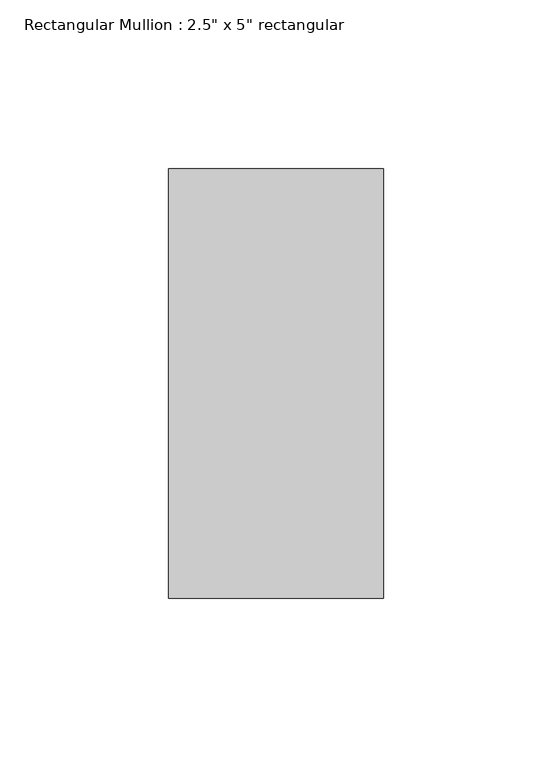
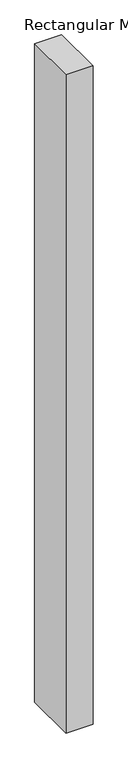
"""IFC4 building model written with IfcOpenShell, lengths in millimetres: member geometry."""

from ifc_helpers import new_model, si_unit, frame, origin, place, context, project, spatial, polyline, outline, extrude, source, transform, mapped, element, save


def member_a798bde5(model_context):
    return source(origin(), model_context, "Body", "SweptSolid", [
        extrude(outline(polyline([(0.0, 63.5), (0.0, -63.5), (-63.5, -63.5), (-63.5, 63.5), (0.0, 63.5)])), frame((0.0, 0.0, -1630.931829), z_axis=(0.0, 0.0, 1.0), x_axis=(1.0, 0.0, 0.0)), (0.0, 0.0, 1.0), 1630.931829),
    ])


if __name__ == "__main__":
    model = new_model("IFC4")
    model_context = context("Model", 3, world=origin())
    ifc_project = project(units=[si_unit("LENGTHUNIT", "METRE", prefix="MILLI")], contexts=[model_context])
    site = spatial("IfcSite", under=ifc_project)
    building = spatial("IfcBuilding", under=site)
    placement = place(None, origin())
    member_shape = member_a798bde5(model_context)
    element("IfcMember", 1, ObjectType="Rectangular Mullion : 2.5\" x 5\" rectangular", at=placement, inside=building, context=model_context, shape_type="MappedRepresentation", body=[
        mapped(member_shape, transform((0.0, 0.0, 0.0), x_axis=(1.0, 0.0, 0.0), y_axis=(0.0, 1.0, 0.0), z_axis=(0.0, 0.0, 1.0))),
    ])
    save(model, "model.ifc")

# Revit data of these elements
# Type "Rectangular Mullion : 2.5\" x 5\" rectangular"
#   built-in parameter 1007304 = 0.416667 (stored number, unit not read)
#   built-in parameter 1007301 = 0.104167 (stored number, unit not read)
#   built-in parameter 1007300 = 0.104167 (stored number, unit not read)
# Element 1 (IfcMember, "Rectangular Mullion : 2.5\" x 5\" rectangular")
#   Materials on its faces: "Aluminum"
# Materials
#   "Aluminum": class "Metal", colour RGB 247 247 247, transparency 0, Description = "Aluminum 6061", Cost = 0
